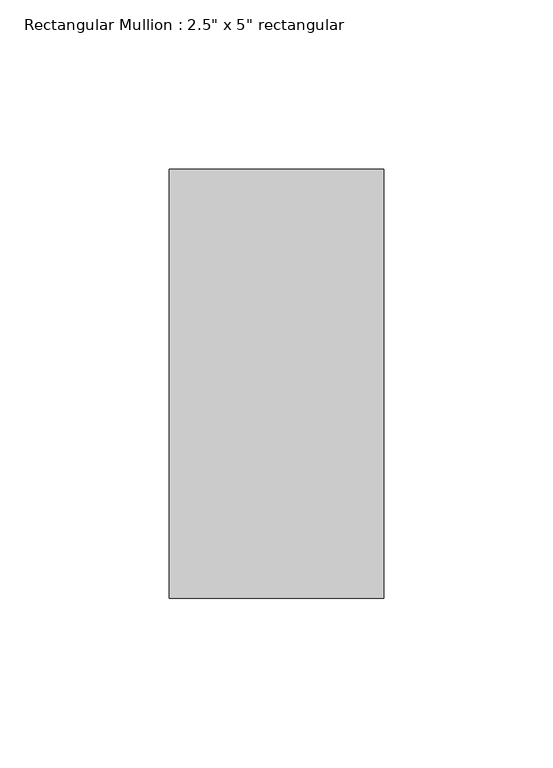
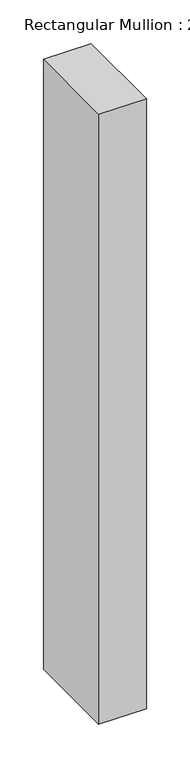
"""IFC4 building model written with IfcOpenShell, lengths in millimetres: member geometry."""

from ifc_helpers import new_model, si_unit, frame, origin, place, context, project, spatial, polyline, outline, extrude, source, transform, mapped, element, save


def member_7bbb9eab(model_context):
    return source(origin(), model_context, "Body", "SweptSolid", [
        extrude(outline(polyline([(31.75, 63.5), (31.75, -63.5), (-31.75, -63.5), (-31.75, 63.5), (31.75, 63.5)])), frame((0.0, 0.0, -854.843224), z_axis=(0.0, 0.0, 1.0), x_axis=(1.0, 0.0, 0.0)), (0.0, 0.0, 1.0), 854.843224),
    ])


if __name__ == "__main__":
    model = new_model("IFC4")
    model_context = context("Model", 3, world=origin())
    ifc_project = project(units=[si_unit("LENGTHUNIT", "METRE", prefix="MILLI")], contexts=[model_context])
    site = spatial("IfcSite", under=ifc_project)
    building = spatial("IfcBuilding", under=site)
    placement = place(None, origin())
    member_shape = member_7bbb9eab(model_context)
    element("IfcMember", 1, ObjectType="Rectangular Mullion : 2.5\" x 5\" rectangular", at=placement, inside=building, context=model_context, shape_type="MappedRepresentation", body=[
        mapped(member_shape, transform((0.0, 0.0, 0.0), x_axis=(1.0, 0.0, 0.0), y_axis=(0.0, 1.0, 0.0), z_axis=(0.0, 0.0, 1.0))),
    ])
    save(model, "model.ifc")

# Revit data of these elements
# Type "Rectangular Mullion : 2.5\" x 5\" rectangular"
#   built-in parameter 1007304 = 0.416667 (stored number, unit not read)
#   built-in parameter 1007301 = 0.104167 (stored number, unit not read)
#   built-in parameter 1007300 = 0.104167 (stored number, unit not read)
# Element 1 (IfcMember, "Rectangular Mullion : 2.5\" x 5\" rectangular")
#   Materials on its faces: "Aluminum"
# Materials
#   "Aluminum": class "Metal", colour RGB 247 247 247, transparency 0, Description = "Aluminum 6061", Cost = 0
